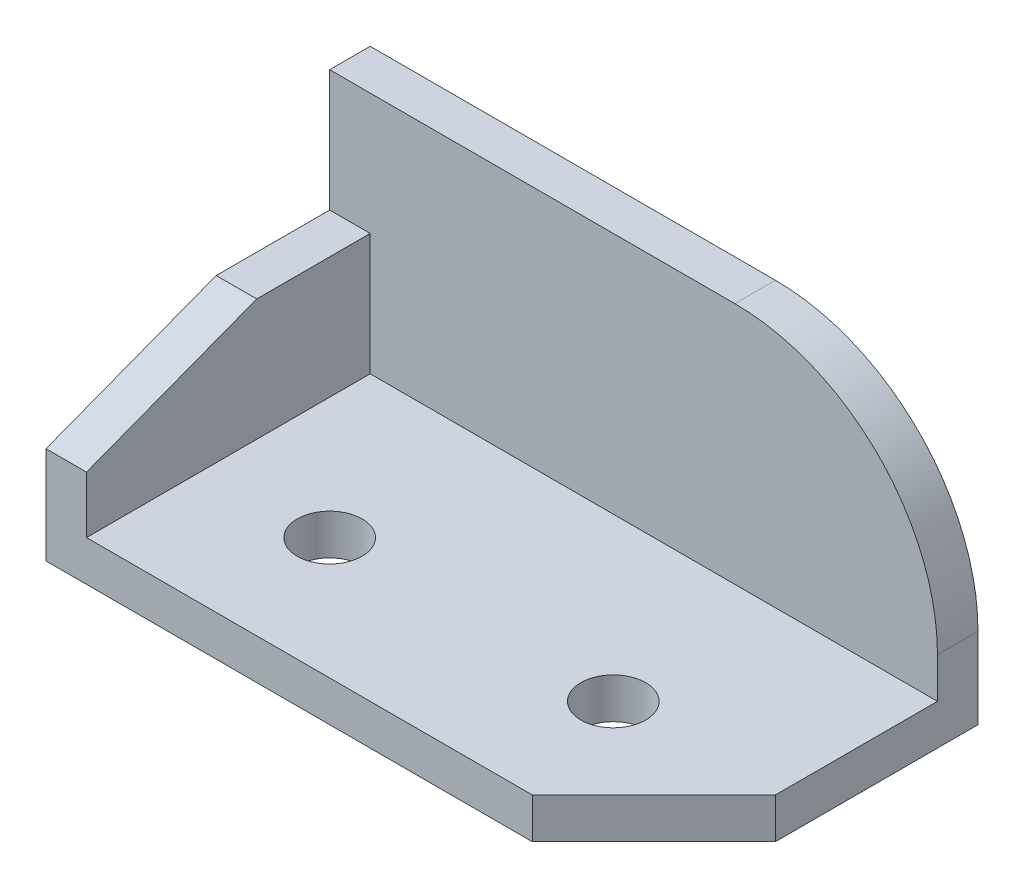
ISO-10303-21;
HEADER;
FILE_DESCRIPTION(('STEP AP214'),'2;1');
FILE_NAME('part.step','',(''),(''),'','','');
FILE_SCHEMA(('AUTOMOTIVE_DESIGN { 1 0 10303 214 1 1 1 1 }'));
ENDSEC;
DATA;
#1=APPLICATION_CONTEXT('core data for automotive mechanical design processes');
#2=APPLICATION_PROTOCOL_DEFINITION('international standard','automotive_design',2000,#1);
#3=PRODUCT_CONTEXT('',#1,'mechanical');
#4=PRODUCT('Part','Part','',(#3));
#5=PRODUCT_RELATED_PRODUCT_CATEGORY('part','',(#4));
#6=PRODUCT_DEFINITION_FORMATION('','',#4);
#7=PRODUCT_DEFINITION_CONTEXT('part definition',#1,'design');
#8=PRODUCT_DEFINITION('design','',#6,#7);
#9=PRODUCT_DEFINITION_SHAPE('','',#8);
#10=(LENGTH_UNIT() NAMED_UNIT(*) SI_UNIT(.MILLI.,.METRE.));
#11=(NAMED_UNIT(*) PLANE_ANGLE_UNIT() SI_UNIT($,.RADIAN.));
#12=(NAMED_UNIT(*) SI_UNIT($,.STERADIAN.) SOLID_ANGLE_UNIT());
#13=UNCERTAINTY_MEASURE_WITH_UNIT(LENGTH_MEASURE(1.E-05),#10,'distance_accuracy_value','');
#14=(GEOMETRIC_REPRESENTATION_CONTEXT(3) GLOBAL_UNCERTAINTY_ASSIGNED_CONTEXT((#13)) GLOBAL_UNIT_ASSIGNED_CONTEXT((#10,
#11,#12)) REPRESENTATION_CONTEXT('',''));
#15=CARTESIAN_POINT('',(0.,0.,0.));
#16=DIRECTION('',(0.,0.,1.));
#17=DIRECTION('',(1.,0.,0.));
#18=AXIS2_PLACEMENT_3D('',#15,#16,#17);
#19=CARTESIAN_POINT('',(75.,5.,0.));
#20=DIRECTION('',(-1.,0.,0.));
#21=DIRECTION('',(0.,0.,1.));
#22=AXIS2_PLACEMENT_3D('',#19,#20,#21);
#23=PLANE('',#22);
#24=DIRECTION('',(0.,0.,1.));
#25=VECTOR('',#24,1.);
#26=CARTESIAN_POINT('',(75.,9.99999999999982,-25.));
#27=LINE('',#26,#25);
#28=CARTESIAN_POINT('',(75.,9.99999999999982,0.));
#29=VERTEX_POINT('',#28);
#30=CARTESIAN_POINT('',(75.,9.99999999999982,5.));
#31=VERTEX_POINT('',#30);
#32=EDGE_CURVE('E132',#29,#31,#27,.T.);
#33=ORIENTED_EDGE('',*,*,#32,.T.);
#34=DIRECTION('',(0.,-1.,0.));
#35=VECTOR('',#34,1.);
#36=CARTESIAN_POINT('',(75.,35.,5.));
#37=LINE('',#36,#35);
#38=CARTESIAN_POINT('',(75.,5.,5.));
#39=VERTEX_POINT('',#38);
#40=EDGE_CURVE('E131',#31,#39,#37,.T.);
#41=ORIENTED_EDGE('',*,*,#40,.T.);
#42=DIRECTION('',(0.,0.,-1.));
#43=VECTOR('',#42,1.);
#44=CARTESIAN_POINT('',(75.,5.,0.));
#45=LINE('',#44,#43);
#46=CARTESIAN_POINT('',(75.,5.,25.));
#47=VERTEX_POINT('',#46);
#48=EDGE_CURVE('E189',#47,#39,#45,.T.);
#49=ORIENTED_EDGE('',*,*,#48,.F.);
#50=DIRECTION('',(0.,-1.,0.));
#51=VECTOR('',#50,1.);
#52=CARTESIAN_POINT('',(75.,5.,25.));
#53=LINE('',#52,#51);
#54=CARTESIAN_POINT('',(75.,0.,25.));
#55=VERTEX_POINT('',#54);
#56=EDGE_CURVE('E208',#47,#55,#53,.T.);
#57=ORIENTED_EDGE('',*,*,#56,.T.);
#58=DIRECTION('',(0.,0.,-1.));
#59=VECTOR('',#58,1.);
#60=CARTESIAN_POINT('',(75.,0.,0.));
#61=LINE('',#60,#59);
#62=CARTESIAN_POINT('',(75.,0.,0.));
#63=VERTEX_POINT('',#62);
#64=EDGE_CURVE('E199',#55,#63,#61,.T.);
#65=ORIENTED_EDGE('',*,*,#64,.T.);
#66=DIRECTION('',(0.,-1.,0.));
#67=VECTOR('',#66,1.);
#68=CARTESIAN_POINT('',(75.,5.,0.));
#69=LINE('',#68,#67);
#70=EDGE_CURVE('E206',#29,#63,#69,.T.);
#71=ORIENTED_EDGE('',*,*,#70,.F.);
#72=EDGE_LOOP('',(#33,#41,#49,#57,#65,#71));
#73=FACE_BOUND('',#72,.T.);
#74=ADVANCED_FACE('F39',(#73),#23,.F.);
#75=CARTESIAN_POINT('',(0.,35.,0.));
#76=DIRECTION('',(0.,1.,0.));
#77=DIRECTION('',(0.,0.,1.));
#78=AXIS2_PLACEMENT_3D('',#75,#76,#77);
#79=PLANE('',#78);
#80=DIRECTION('',(1.,0.,0.));
#81=VECTOR('',#80,1.);
#82=CARTESIAN_POINT('',(0.,35.,5.));
#83=LINE('',#82,#81);
#84=CARTESIAN_POINT('',(0.,35.,5.));
#85=VERTEX_POINT('',#84);
#86=CARTESIAN_POINT('',(49.9999999999998,35.,5.));
#87=VERTEX_POINT('',#86);
#88=EDGE_CURVE('E128',#85,#87,#83,.T.);
#89=ORIENTED_EDGE('',*,*,#88,.T.);
#90=DIRECTION('',(0.,0.,1.));
#91=VECTOR('',#90,1.);
#92=CARTESIAN_POINT('',(50.,35.,-25.));
#93=LINE('',#92,#91);
#94=CARTESIAN_POINT('',(50.,35.,0.));
#95=VERTEX_POINT('',#94);
#96=EDGE_CURVE('E11',#87,#95,#93,.F.);
#97=ORIENTED_EDGE('',*,*,#96,.T.);
#98=DIRECTION('',(1.,0.,0.));
#99=VECTOR('',#98,1.);
#100=CARTESIAN_POINT('',(0.,35.,0.));
#101=LINE('',#100,#99);
#102=CARTESIAN_POINT('',(0.,35.,0.));
#103=VERTEX_POINT('',#102);
#104=EDGE_CURVE('E139',#103,#95,#101,.T.);
#105=ORIENTED_EDGE('',*,*,#104,.F.);
#106=DIRECTION('',(0.,0.,1.));
#107=VECTOR('',#106,1.);
#108=CARTESIAN_POINT('',(0.,35.,0.));
#109=LINE('',#108,#107);
#110=EDGE_CURVE('E137',#103,#85,#109,.T.);
#111=ORIENTED_EDGE('',*,*,#110,.T.);
#112=EDGE_LOOP('',(#89,#97,#105,#111));
#113=FACE_BOUND('',#112,.T.);
#114=ADVANCED_FACE('F136',(#113),#79,.T.);
#115=CARTESIAN_POINT('',(0.,5.,0.));
#116=DIRECTION('',(0.,1.,0.));
#117=DIRECTION('',(0.,0.,1.));
#118=AXIS2_PLACEMENT_3D('',#115,#116,#117);
#119=PLANE('',#118);
#120=CARTESIAN_POINT('',(20.,5.,25.));
#121=DIRECTION('',(0.,1.,0.));
#122=DIRECTION('',(0.,0.,1.));
#123=AXIS2_PLACEMENT_3D('',#120,#121,#122);
#124=CIRCLE('',#123,4.);
#125=CARTESIAN_POINT('',(20.,5.,29.));
#126=VERTEX_POINT('',#125);
#127=EDGE_CURVE('E178',#126,#126,#124,.T.);
#128=ORIENTED_EDGE('',*,*,#127,.F.);
#129=EDGE_LOOP('',(#128));
#130=FACE_BOUND('',#129,.T.);
#131=CARTESIAN_POINT('',(55.,5.,25.));
#132=DIRECTION('',(0.,1.,0.));
#133=DIRECTION('',(0.,0.,1.));
#134=AXIS2_PLACEMENT_3D('',#131,#132,#133);
#135=CIRCLE('',#134,4.);
#136=CARTESIAN_POINT('',(55.,5.,29.));
#137=VERTEX_POINT('',#136);
#138=EDGE_CURVE('E171',#137,#137,#135,.T.);
#139=ORIENTED_EDGE('',*,*,#138,.F.);
#140=EDGE_LOOP('',(#139));
#141=FACE_BOUND('',#140,.T.);
#142=ORIENTED_EDGE('',*,*,#48,.T.);
#143=DIRECTION('',(1.,0.,0.));
#144=VECTOR('',#143,1.);
#145=CARTESIAN_POINT('',(0.,5.,5.));
#146=LINE('',#145,#144);
#147=CARTESIAN_POINT('',(5.,5.,5.));
#148=VERTEX_POINT('',#147);
#149=EDGE_CURVE('E141',#148,#39,#146,.T.);
#150=ORIENTED_EDGE('',*,*,#149,.F.);
#151=DIRECTION('',(0.,0.,-1.));
#152=VECTOR('',#151,1.);
#153=CARTESIAN_POINT('',(5.,5.,0.));
#154=LINE('',#153,#152);
#155=CARTESIAN_POINT('',(5.,5.,40.));
#156=VERTEX_POINT('',#155);
#157=EDGE_CURVE('E170',#156,#148,#154,.T.);
#158=ORIENTED_EDGE('',*,*,#157,.F.);
#159=DIRECTION('',(1.,0.,0.));
#160=VECTOR('',#159,1.);
#161=CARTESIAN_POINT('',(0.,5.,40.));
#162=LINE('',#161,#160);
#163=CARTESIAN_POINT('',(60.,5.,40.));
#164=VERTEX_POINT('',#163);
#165=EDGE_CURVE('E183',#156,#164,#162,.T.);
#166=ORIENTED_EDGE('',*,*,#165,.T.);
#167=DIRECTION('',(0.707106781186547,0.,-0.707106781186548));
#168=VECTOR('',#167,1.);
#169=CARTESIAN_POINT('',(60.,5.,40.));
#170=LINE('',#169,#168);
#171=EDGE_CURVE('E190',#164,#47,#170,.T.);
#172=ORIENTED_EDGE('',*,*,#171,.T.);
#173=EDGE_LOOP('',(#142,#150,#158,#166,#172));
#174=FACE_BOUND('',#173,.T.);
#175=ADVANCED_FACE('F233',(#130,#141,#174),#119,.T.);
#176=CARTESIAN_POINT('',(5.,25.,0.));
#177=DIRECTION('',(-1.,0.,0.));
#178=DIRECTION('',(0.,0.,1.));
#179=AXIS2_PLACEMENT_3D('',#176,#177,#178);
#180=PLANE('',#179);
#181=DIRECTION('',(0.,-1.,0.));
#182=VECTOR('',#181,1.);
#183=CARTESIAN_POINT('',(5.,25.,5.));
#184=LINE('',#183,#182);
#185=CARTESIAN_POINT('',(5.,20.,5.));
#186=VERTEX_POINT('',#185);
#187=EDGE_CURVE('E151',#186,#148,#184,.T.);
#188=ORIENTED_EDGE('',*,*,#187,.F.);
#189=DIRECTION('',(0.,0.,-1.));
#190=VECTOR('',#189,1.);
#191=CARTESIAN_POINT('',(5.,20.,19.));
#192=LINE('',#191,#190);
#193=CARTESIAN_POINT('',(5.,20.,19.));
#194=VERTEX_POINT('',#193);
#195=EDGE_CURVE('E154',#194,#186,#192,.T.);
#196=ORIENTED_EDGE('',*,*,#195,.F.);
#197=DIRECTION('',(0.,0.355995327591988,-0.934487734928968));
#198=VECTOR('',#197,1.);
#199=CARTESIAN_POINT('',(5.,20.,19.));
#200=LINE('',#199,#198);
#201=CARTESIAN_POINT('',(5.00000000000001,12.,40.));
#202=VERTEX_POINT('',#201);
#203=EDGE_CURVE('E153',#202,#194,#200,.T.);
#204=ORIENTED_EDGE('',*,*,#203,.F.);
#205=DIRECTION('',(0.,-1.,0.));
#206=VECTOR('',#205,1.);
#207=CARTESIAN_POINT('',(5.00000000000001,25.,40.));
#208=LINE('',#207,#206);
#209=EDGE_CURVE('E168',#202,#156,#208,.T.);
#210=ORIENTED_EDGE('',*,*,#209,.T.);
#211=ORIENTED_EDGE('',*,*,#157,.T.);
#212=EDGE_LOOP('',(#188,#196,#204,#210,#211));
#213=FACE_BOUND('',#212,.T.);
#214=ADVANCED_FACE('F222',(#213),#180,.F.);
#215=CARTESIAN_POINT('',(-15.,20.,19.));
#216=DIRECTION('',(0.,-1.,0.));
#217=DIRECTION('',(0.,0.,-1.));
#218=AXIS2_PLACEMENT_3D('',#215,#216,#217);
#219=PLANE('',#218);
#220=DIRECTION('',(1.,0.,0.));
#221=VECTOR('',#220,1.);
#222=CARTESIAN_POINT('',(-15.,20.,5.));
#223=LINE('',#222,#221);
#224=CARTESIAN_POINT('',(0.,20.,5.));
#225=VERTEX_POINT('',#224);
#226=EDGE_CURVE('E50',#225,#186,#223,.T.);
#227=ORIENTED_EDGE('',*,*,#226,.F.);
#228=DIRECTION('',(0.,0.,-1.));
#229=VECTOR('',#228,1.);
#230=CARTESIAN_POINT('',(0.,20.,0.));
#231=LINE('',#230,#229);
#232=CARTESIAN_POINT('',(0.,20.,19.));
#233=VERTEX_POINT('',#232);
#234=EDGE_CURVE('E163',#233,#225,#231,.T.);
#235=ORIENTED_EDGE('',*,*,#234,.F.);
#236=DIRECTION('',(1.,0.,0.));
#237=VECTOR('',#236,1.);
#238=CARTESIAN_POINT('',(-15.,20.,19.));
#239=LINE('',#238,#237);
#240=EDGE_CURVE('E158',#233,#194,#239,.T.);
#241=ORIENTED_EDGE('',*,*,#240,.T.);
#242=ORIENTED_EDGE('',*,*,#195,.T.);
#243=EDGE_LOOP('',(#227,#235,#241,#242));
#244=FACE_BOUND('',#243,.T.);
#245=ADVANCED_FACE('F224',(#244),#219,.F.);
#246=CARTESIAN_POINT('',(0.,0.,0.));
#247=DIRECTION('',(0.,1.,0.));
#248=DIRECTION('',(0.,0.,1.));
#249=AXIS2_PLACEMENT_3D('',#246,#247,#248);
#250=PLANE('',#249);
#251=DIRECTION('',(0.,0.,1.));
#252=VECTOR('',#251,1.);
#253=CARTESIAN_POINT('',(0.,0.,0.));
#254=LINE('',#253,#252);
#255=CARTESIAN_POINT('',(0.,0.,0.));
#256=VERTEX_POINT('',#255);
#257=CARTESIAN_POINT('',(0.,0.,40.));
#258=VERTEX_POINT('',#257);
#259=EDGE_CURVE('E185',#256,#258,#254,.T.);
#260=ORIENTED_EDGE('',*,*,#259,.F.);
#261=DIRECTION('',(-1.,0.,0.));
#262=VECTOR('',#261,1.);
#263=CARTESIAN_POINT('',(0.,0.,0.));
#264=LINE('',#263,#262);
#265=EDGE_CURVE('E186',#63,#256,#264,.T.);
#266=ORIENTED_EDGE('',*,*,#265,.F.);
#267=ORIENTED_EDGE('',*,*,#64,.F.);
#268=DIRECTION('',(0.707106781186547,0.,-0.707106781186548));
#269=VECTOR('',#268,1.);
#270=CARTESIAN_POINT('',(60.,0.,40.));
#271=LINE('',#270,#269);
#272=CARTESIAN_POINT('',(60.,0.,40.));
#273=VERTEX_POINT('',#272);
#274=EDGE_CURVE('E196',#273,#55,#271,.T.);
#275=ORIENTED_EDGE('',*,*,#274,.F.);
#276=DIRECTION('',(1.,0.,0.));
#277=VECTOR('',#276,1.);
#278=CARTESIAN_POINT('',(0.,0.,40.));
#279=LINE('',#278,#277);
#280=EDGE_CURVE('E198',#258,#273,#279,.T.);
#281=ORIENTED_EDGE('',*,*,#280,.F.);
#282=EDGE_LOOP('',(#260,#266,#267,#275,#281));
#283=FACE_BOUND('',#282,.T.);
#284=CARTESIAN_POINT('',(20.,0.,25.));
#285=DIRECTION('',(0.,1.,0.));
#286=DIRECTION('',(0.,0.,1.));
#287=AXIS2_PLACEMENT_3D('',#284,#285,#286);
#288=CIRCLE('',#287,4.);
#289=CARTESIAN_POINT('',(20.,0.,29.));
#290=VERTEX_POINT('',#289);
#291=EDGE_CURVE('E176',#290,#290,#288,.T.);
#292=ORIENTED_EDGE('',*,*,#291,.T.);
#293=EDGE_LOOP('',(#292));
#294=FACE_BOUND('',#293,.T.);
#295=CARTESIAN_POINT('',(55.,0.,25.));
#296=DIRECTION('',(0.,1.,0.));
#297=DIRECTION('',(0.,0.,1.));
#298=AXIS2_PLACEMENT_3D('',#295,#296,#297);
#299=CIRCLE('',#298,4.);
#300=CARTESIAN_POINT('',(55.,0.,29.));
#301=VERTEX_POINT('',#300);
#302=EDGE_CURVE('E175',#301,#301,#299,.T.);
#303=ORIENTED_EDGE('',*,*,#302,.T.);
#304=EDGE_LOOP('',(#303));
#305=FACE_BOUND('',#304,.T.);
#306=ADVANCED_FACE('F248',(#283,#294,#305),#250,.F.);
#307=CARTESIAN_POINT('',(0.,5.,0.));
#308=DIRECTION('',(1.,0.,0.));
#309=DIRECTION('',(0.,0.,-1.));
#310=AXIS2_PLACEMENT_3D('',#307,#308,#309);
#311=PLANE('',#310);
#312=ORIENTED_EDGE('',*,*,#234,.T.);
#313=DIRECTION('',(0.,-1.,0.));
#314=VECTOR('',#313,1.);
#315=CARTESIAN_POINT('',(0.,35.,5.));
#316=LINE('',#315,#314);
#317=EDGE_CURVE('E149',#85,#225,#316,.T.);
#318=ORIENTED_EDGE('',*,*,#317,.F.);
#319=ORIENTED_EDGE('',*,*,#110,.F.);
#320=DIRECTION('',(0.,-1.,0.));
#321=VECTOR('',#320,1.);
#322=CARTESIAN_POINT('',(0.,5.,0.));
#323=LINE('',#322,#321);
#324=EDGE_CURVE('E192',#103,#256,#323,.T.);
#325=ORIENTED_EDGE('',*,*,#324,.T.);
#326=ORIENTED_EDGE('',*,*,#259,.T.);
#327=DIRECTION('',(0.,-1.,0.));
#328=VECTOR('',#327,1.);
#329=CARTESIAN_POINT('',(0.,5.,40.));
#330=LINE('',#329,#328);
#331=CARTESIAN_POINT('',(0.,12.,40.));
#332=VERTEX_POINT('',#331);
#333=EDGE_CURVE('E212',#332,#258,#330,.T.);
#334=ORIENTED_EDGE('',*,*,#333,.F.);
#335=DIRECTION('',(0.,0.355995327591988,-0.934487734928968));
#336=VECTOR('',#335,1.);
#337=CARTESIAN_POINT('',(0.,24.419801980198,7.3980198019802));
#338=LINE('',#337,#336);
#339=EDGE_CURVE('E159',#332,#233,#338,.T.);
#340=ORIENTED_EDGE('',*,*,#339,.T.);
#341=EDGE_LOOP('',(#312,#318,#319,#325,#326,#334,#340));
#342=FACE_BOUND('',#341,.T.);
#343=ADVANCED_FACE('F41',(#342),#311,.F.);
#344=CARTESIAN_POINT('',(0.,5.,40.));
#345=DIRECTION('',(0.,0.,-1.));
#346=DIRECTION('',(-1.,0.,0.));
#347=AXIS2_PLACEMENT_3D('',#344,#345,#346);
#348=PLANE('',#347);
#349=ORIENTED_EDGE('',*,*,#209,.F.);
#350=DIRECTION('',(1.,0.,0.));
#351=VECTOR('',#350,1.);
#352=CARTESIAN_POINT('',(-15.,12.,40.));
#353=LINE('',#352,#351);
#354=EDGE_CURVE('E63',#332,#202,#353,.T.);
#355=ORIENTED_EDGE('',*,*,#354,.F.);
#356=ORIENTED_EDGE('',*,*,#333,.T.);
#357=ORIENTED_EDGE('',*,*,#280,.T.);
#358=DIRECTION('',(0.,-1.,0.));
#359=VECTOR('',#358,1.);
#360=CARTESIAN_POINT('',(60.,5.,40.));
#361=LINE('',#360,#359);
#362=EDGE_CURVE('E211',#164,#273,#361,.T.);
#363=ORIENTED_EDGE('',*,*,#362,.F.);
#364=ORIENTED_EDGE('',*,*,#165,.F.);
#365=EDGE_LOOP('',(#349,#355,#356,#357,#363,#364));
#366=FACE_BOUND('',#365,.T.);
#367=ADVANCED_FACE('F227',(#366),#348,.F.);
#368=CARTESIAN_POINT('',(60.,5.,40.));
#369=DIRECTION('',(-0.707106781186548,0.,-0.707106781186547));
#370=DIRECTION('',(-0.707106781186547,0.,0.707106781186548));
#371=AXIS2_PLACEMENT_3D('',#368,#369,#370);
#372=PLANE('',#371);
#373=ORIENTED_EDGE('',*,*,#274,.T.);
#374=ORIENTED_EDGE('',*,*,#56,.F.);
#375=ORIENTED_EDGE('',*,*,#171,.F.);
#376=ORIENTED_EDGE('',*,*,#362,.T.);
#377=EDGE_LOOP('',(#373,#374,#375,#376));
#378=FACE_BOUND('',#377,.T.);
#379=ADVANCED_FACE('F252',(#378),#372,.F.);
#380=CARTESIAN_POINT('',(0.,5.,0.));
#381=DIRECTION('',(0.,0.,1.));
#382=DIRECTION('',(1.,0.,0.));
#383=AXIS2_PLACEMENT_3D('',#380,#381,#382);
#384=PLANE('',#383);
#385=ORIENTED_EDGE('',*,*,#104,.T.);
#386=CARTESIAN_POINT('',(50.,10.,0.));
#387=DIRECTION('',(0.,0.,1.));
#388=DIRECTION('',(1.,0.,0.));
#389=AXIS2_PLACEMENT_3D('',#386,#387,#388);
#390=CIRCLE('',#389,25.);
#391=EDGE_CURVE('E53',#95,#29,#390,.F.);
#392=ORIENTED_EDGE('',*,*,#391,.T.);
#393=ORIENTED_EDGE('',*,*,#70,.T.);
#394=ORIENTED_EDGE('',*,*,#265,.T.);
#395=ORIENTED_EDGE('',*,*,#324,.F.);
#396=EDGE_LOOP('',(#385,#392,#393,#394,#395));
#397=FACE_BOUND('',#396,.T.);
#398=ADVANCED_FACE('F245',(#397),#384,.F.);
#399=CARTESIAN_POINT('',(20.,5.,25.));
#400=DIRECTION('',(0.,-1.,0.));
#401=DIRECTION('',(0.,0.,-1.));
#402=AXIS2_PLACEMENT_3D('',#399,#400,#401);
#403=CYLINDRICAL_SURFACE('',#402,4.);
#404=ORIENTED_EDGE('',*,*,#127,.T.);
#405=EDGE_LOOP('',(#404));
#406=FACE_BOUND('',#405,.T.);
#407=ORIENTED_EDGE('',*,*,#291,.F.);
#408=EDGE_LOOP('',(#407));
#409=FACE_BOUND('',#408,.T.);
#410=ADVANCED_FACE('F257',(#406,#409),#403,.F.);
#411=CARTESIAN_POINT('',(55.,5.,25.));
#412=DIRECTION('',(0.,-1.,0.));
#413=DIRECTION('',(0.,0.,-1.));
#414=AXIS2_PLACEMENT_3D('',#411,#412,#413);
#415=CYLINDRICAL_SURFACE('',#414,4.);
#416=ORIENTED_EDGE('',*,*,#138,.T.);
#417=EDGE_LOOP('',(#416));
#418=FACE_BOUND('',#417,.T.);
#419=ORIENTED_EDGE('',*,*,#302,.F.);
#420=EDGE_LOOP('',(#419));
#421=FACE_BOUND('',#420,.T.);
#422=ADVANCED_FACE('F277',(#418,#421),#415,.F.);
#423=CARTESIAN_POINT('',(-15.,20.,19.));
#424=DIRECTION('',(0.,-0.934487734928968,-0.355995327591988));
#425=DIRECTION('',(0.,0.355995327591988,-0.934487734928968));
#426=AXIS2_PLACEMENT_3D('',#423,#424,#425);
#427=PLANE('',#426);
#428=ORIENTED_EDGE('',*,*,#354,.T.);
#429=ORIENTED_EDGE('',*,*,#203,.T.);
#430=ORIENTED_EDGE('',*,*,#240,.F.);
#431=ORIENTED_EDGE('',*,*,#339,.F.);
#432=EDGE_LOOP('',(#428,#429,#430,#431));
#433=FACE_BOUND('',#432,.T.);
#434=ADVANCED_FACE('F223',(#433),#427,.F.);
#435=CARTESIAN_POINT('',(0.,35.,5.));
#436=DIRECTION('',(0.,0.,-1.));
#437=DIRECTION('',(-1.,0.,0.));
#438=AXIS2_PLACEMENT_3D('',#435,#436,#437);
#439=PLANE('',#438);
#440=ORIENTED_EDGE('',*,*,#40,.F.);
#441=CARTESIAN_POINT('',(50.,10.,5.));
#442=DIRECTION('',(0.,0.,-1.));
#443=DIRECTION('',(1.,0.,0.));
#444=AXIS2_PLACEMENT_3D('',#441,#442,#443);
#445=CIRCLE('',#444,25.);
#446=EDGE_CURVE('E121',#87,#31,#445,.T.);
#447=ORIENTED_EDGE('',*,*,#446,.F.);
#448=ORIENTED_EDGE('',*,*,#88,.F.);
#449=ORIENTED_EDGE('',*,*,#317,.T.);
#450=ORIENTED_EDGE('',*,*,#226,.T.);
#451=ORIENTED_EDGE('',*,*,#187,.T.);
#452=ORIENTED_EDGE('',*,*,#149,.T.);
#453=EDGE_LOOP('',(#440,#447,#448,#449,#450,#451,#452));
#454=FACE_BOUND('',#453,.T.);
#455=ADVANCED_FACE('F129',(#454),#439,.F.);
#456=CARTESIAN_POINT('',(50.,10.,-25.));
#457=DIRECTION('',(0.,0.,1.));
#458=DIRECTION('',(1.,0.,0.));
#459=AXIS2_PLACEMENT_3D('',#456,#457,#458);
#460=CYLINDRICAL_SURFACE('',#459,25.);
#461=ORIENTED_EDGE('',*,*,#96,.F.);
#462=ORIENTED_EDGE('',*,*,#446,.T.);
#463=ORIENTED_EDGE('',*,*,#32,.F.);
#464=ORIENTED_EDGE('',*,*,#391,.F.);
#465=EDGE_LOOP('',(#461,#462,#463,#464));
#466=FACE_BOUND('',#465,.T.);
#467=ADVANCED_FACE('F119',(#466),#460,.T.);
#468=CLOSED_SHELL('',(#74,#114,#175,#214,#245,#306,#343,#367,#379,#398,#410,#422,#434,#455,#467));
#469=MANIFOLD_SOLID_BREP('B2',#468);
#470=ADVANCED_BREP_SHAPE_REPRESENTATION('',(#18,#469),#14);
#471=SHAPE_DEFINITION_REPRESENTATION(#9,#470);
ENDSEC;
END-ISO-10303-21;
